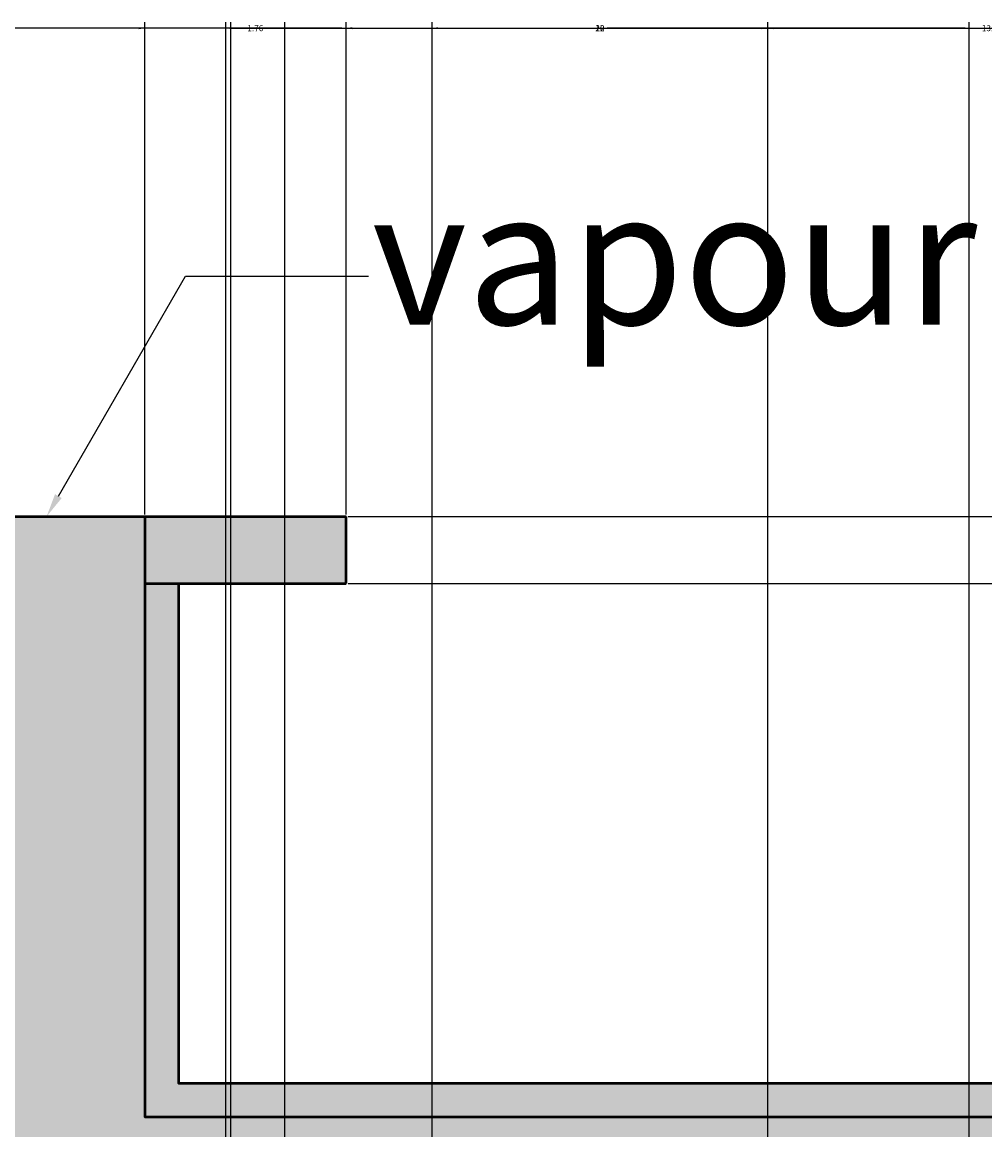
# Model space of a CAD drawing. Units: inches. Extents: x -12 to 334, y -10 to 186.
# Tile 67 of 77: x 210 to 239, y 137 to 170. Entities that reach past the tile are written whole.
import ezdxf
from ezdxf import colors
from ezdxf.entities.mleader import LeaderData, LeaderLine
from ezdxf.math import Vec2, Vec3

# ---------------------------------------------------------------- set-up
doc = ezdxf.new("R2010")
doc.units = ezdxf.units.IN
doc.header["$MEASUREMENT"] = 0
for name, color, linetype, lineweight in [('M-ANNO-TEXT', 3, 'Continuous', 25), ('M-DIMS', 2, 'Continuous', 18), ('M-EQPM', 7, 'Continuous', 50), ('M-EQPM-PATT', 8, 'Continuous', 18)]:
    doc.layers.add(name, color=color, linetype=linetype, lineweight=lineweight)
doc.styles.get("Standard").update_dxf_attribs({"font": 'arial.ttf'})
doc.dimstyles.get("Standard").update_dxf_attribs({"dimtxt": 0.18, "dimasz": 0.18, "dimexe": 0.18, "dimexo": 0.0625, "dimgap": 0.09, "dimtad": 0, "dimtih": 1, "dimtoh": 1, "dimdec": 4, "dimzin": 0, "dimdsep": 46, "dimtxsty": 'Standard', "dimcen": 0.09, "dimadec": 0, "dimazin": 0, "dimtfac": 1, "dimtdec": 4, "dimtofl": 0, "dimtmove": 0, "dimatfit": 3, "dimfxl": 1, "dimtolj": 1, "dimtzin": 0, "dimarcsym": 0})

# ---------------------------------------------------------------- blocks, each defined once
blk = doc.blocks.new('*D19')
at = {"layer": 'Defpoints', "color": 0, "transparency": 16777216}
for p in [(220.017, 169.385), (190.342, 154.835), (220.017, 154.835)]:
    blk.add_point(p, dxfattribs=at)
at = {"layer": 'M-DIMS', "color": 0, "lineweight": -2, "transparency": 16777216}
for p, q in [((190.342, 154.897), (190.342, 169.565)), ((190.522, 169.385), (204.714, 169.385)), ((219.837, 169.385), (205.645, 169.385)), ((220.017, 154.897), (220.017, 169.565))]:
    blk.add_line(p, q, dxfattribs=at)
at = {"layer": 'M-DIMS', "color": 0, "transparency": 16777216}
for points in [[(190.522, 169.415), (190.522, 169.355), (190.342, 169.385)], [(219.837, 169.415), (219.837, 169.355), (220.017, 169.385)]]:
    blk.add_solid(points, dxfattribs=at)
at = {"layer": 'M-DIMS', "color": 0, "transparency": 16777216, "insert": (205.179, 169.385), "char_height": 0.18, "attachment_point": 5}
blk.add_mtext('\\A1;29.675', dxfattribs=at)
blk = doc.blocks.new('*D20')
at = {"layer": 'Defpoints', "color": 0, "transparency": 16777216}
for p in [(214.017, 169.385), (196.342, 154.835), (214.017, 154.835)]:
    blk.add_point(p, dxfattribs=at)
at = {"layer": 'M-DIMS', "color": 0, "lineweight": -2, "transparency": 16777216}
for p, q in [((196.342, 154.897), (196.342, 169.565)), ((196.522, 169.385), (204.724, 169.385)), ((213.837, 169.385), (205.635, 169.385)), ((214.017, 154.897), (214.017, 169.565))]:
    blk.add_line(p, q, dxfattribs=at)
at = {"layer": 'M-DIMS', "color": 0, "transparency": 16777216}
for points in [[(196.522, 169.415), (196.522, 169.355), (196.342, 169.385)], [(213.837, 169.415), (213.837, 169.355), (214.017, 169.385)]]:
    blk.add_solid(points, dxfattribs=at)
at = {"layer": 'M-DIMS', "color": 0, "transparency": 16777216, "insert": (205.179, 169.385), "char_height": 0.18, "attachment_point": 5}
blk.add_mtext('\\A1;17.675', dxfattribs=at)
blk = doc.blocks.new('*D21')
at = {"layer": 'Defpoints', "color": 0, "transparency": 16777216}
for p in [(269.381, 169.385), (220.017, 154.835), (269.381, 137.943)]:
    blk.add_point(p, dxfattribs=at)
at = {"layer": 'M-DIMS', "color": 0, "lineweight": -2, "transparency": 16777216}
for p, q in [((220.017, 154.897), (220.017, 169.565)), ((220.197, 169.385), (244.301, 169.385)), ((269.201, 169.385), (245.096, 169.385)), ((269.381, 138.006), (269.381, 169.565))]:
    blk.add_line(p, q, dxfattribs=at)
at = {"layer": 'M-DIMS', "color": 0, "transparency": 16777216}
for points in [[(220.197, 169.415), (220.197, 169.355), (220.017, 169.385)], [(269.201, 169.415), (269.201, 169.355), (269.381, 169.385)]]:
    blk.add_solid(points, dxfattribs=at)
at = {"layer": 'M-DIMS', "color": 0, "transparency": 16777216, "insert": (244.699, 169.385), "char_height": 0.18, "attachment_point": 5}
blk.add_mtext('\\A1;49.36', dxfattribs=at)
blk = doc.blocks.new('*D23')
at = {"layer": 'Defpoints', "color": 0, "transparency": 16777216}
for p in [(220.017, 154.835), (220.017, 152.835), (295.976, 152.835)]:
    blk.add_point(p, dxfattribs=at)
at = {"layer": 'M-DIMS', "color": 0, "lineweight": -2, "transparency": 16777216}
for p, q in [((220.079, 154.835), (296.156, 154.835)), ((295.976, 154.655), (295.976, 154.015)), ((295.976, 153.015), (295.976, 153.654)), ((220.079, 152.835), (296.156, 152.835))]:
    blk.add_line(p, q, dxfattribs=at)
at = {"layer": 'M-DIMS', "color": 0, "transparency": 16777216}
for points in [[(295.946, 154.655), (296.006, 154.655), (295.976, 154.835)], [(295.946, 153.015), (296.006, 153.015), (295.976, 152.835)]]:
    blk.add_solid(points, dxfattribs=at)
at = {"layer": 'M-DIMS', "color": 0, "transparency": 16777216, "insert": (295.976, 153.835), "char_height": 0.18, "attachment_point": 5}
blk.add_mtext('\\A1;2', dxfattribs=at)
blk = doc.blocks.new('*D27')
at = {"layer": 'Defpoints', "color": 0, "transparency": 16777216}
for p in [(238.576, 169.385), (216.576, 32.854), (238.576, 32.854)]:
    blk.add_point(p, dxfattribs=at)
at = {"layer": 'M-DIMS', "color": 0, "lineweight": -2, "transparency": 16777216}
for p, q in [((216.576, 32.917), (216.576, 169.565)), ((216.756, 169.385), (227.357, 169.385)), ((238.396, 169.385), (227.796, 169.385)), ((238.576, 32.917), (238.576, 169.565))]:
    blk.add_line(p, q, dxfattribs=at)
at = {"layer": 'M-DIMS', "color": 0, "transparency": 16777216}
for points in [[(216.756, 169.415), (216.756, 169.355), (216.576, 169.385)], [(238.396, 169.415), (238.396, 169.355), (238.576, 169.385)]]:
    blk.add_solid(points, dxfattribs=at)
at = {"layer": 'M-DIMS', "color": 0, "transparency": 16777216, "insert": (227.576, 169.385), "char_height": 0.18, "attachment_point": 5}
blk.add_mtext('\\A1;22', dxfattribs=at)
blk = doc.blocks.new('*D28')
at = {"layer": 'Defpoints', "color": 0, "transparency": 16777216}
for p in [(232.576, 169.385), (222.576, 30.854), (232.576, 30.854)]:
    blk.add_point(p, dxfattribs=at)
at = {"layer": 'M-DIMS', "color": 0, "lineweight": -2, "transparency": 16777216}
for p, q in [((222.576, 30.917), (222.576, 169.565)), ((222.756, 169.385), (227.366, 169.385)), ((232.396, 169.385), (227.786, 169.385)), ((232.576, 30.917), (232.576, 169.565))]:
    blk.add_line(p, q, dxfattribs=at)
at = {"layer": 'M-DIMS', "color": 0, "transparency": 16777216}
for points in [[(222.756, 169.415), (222.756, 169.355), (222.576, 169.385)], [(232.396, 169.415), (232.396, 169.355), (232.576, 169.385)]]:
    blk.add_solid(points, dxfattribs=at)
at = {"layer": 'M-DIMS', "color": 0, "transparency": 16777216, "insert": (227.576, 169.385), "char_height": 0.18, "attachment_point": 5}
blk.add_mtext('\\A1;10', dxfattribs=at)
blk = doc.blocks.new('*D34')
at = {"layer": 'Defpoints', "color": 0, "transparency": 16777216}
for p in [(218.192, 169.385), (216.428, 98.108), (218.192, 98.108)]:
    blk.add_point(p, dxfattribs=at)
at = {"layer": 'M-DIMS', "color": 0, "lineweight": -2, "transparency": 16777216}
for p, q in [((216.428, 98.171), (216.428, 169.565)), ((216.608, 169.385), (216.995, 169.385)), ((218.012, 169.385), (217.625, 169.385)), ((218.192, 98.171), (218.192, 169.565))]:
    blk.add_line(p, q, dxfattribs=at)
at = {"layer": 'M-DIMS', "color": 0, "transparency": 16777216}
for points in [[(216.608, 169.415), (216.608, 169.355), (216.428, 169.385)], [(218.012, 169.415), (218.012, 169.355), (218.192, 169.385)]]:
    blk.add_solid(points, dxfattribs=at)
at = {"layer": 'M-DIMS', "color": 0, "transparency": 16777216, "insert": (217.31, 169.385), "char_height": 0.18, "attachment_point": 5}
blk.add_mtext('\\A1;1.76', dxfattribs=at)
blk = doc.blocks.new('*D37')
at = {"layer": 'Defpoints', "color": 0, "transparency": 16777216}
for p in [(245.935, 169.385), (232.576, 46.854), (245.935, 46.854)]:
    blk.add_point(p, dxfattribs=at)
at = {"layer": 'M-DIMS', "color": 0, "lineweight": -2, "transparency": 16777216}
for p, q in [((232.576, 46.917), (232.576, 169.565)), ((232.756, 169.385), (238.871, 169.385)), ((245.755, 169.385), (239.641, 169.385)), ((245.935, 46.917), (245.935, 169.565))]:
    blk.add_line(p, q, dxfattribs=at)
at = {"layer": 'M-DIMS', "color": 0, "transparency": 16777216}
for points in [[(232.756, 169.415), (232.756, 169.355), (232.576, 169.385)], [(245.755, 169.415), (245.755, 169.355), (245.935, 169.385)]]:
    blk.add_solid(points, dxfattribs=at)
at = {"layer": 'M-DIMS', "color": 0, "transparency": 16777216, "insert": (239.256, 169.385), "char_height": 0.18, "attachment_point": 5}
blk.add_mtext('\\A1;13.36', dxfattribs=at)

msp = doc.modelspace()

# ---------------------------------------------------------------- hatches: boundary and pattern name
at = {"layer": 'M-EQPM-PATT', "transparency": 33554556}
h = msp.add_hatch(color=256, dxfattribs=at)
h.set_gradient(color1=(248, 206, 179), color2=(248, 206, 179), tint=1)
h.paths.add_polyline_path([(179.7818, 136.8871), (126.9567, 136.8871), (106.1771, 100.8958), (171.5458, 100.8958)])
h.paths.add_polyline_path([(268.3808, 136.9435), (214.0166, 136.9435), (214.0166, 154.8345), (196.3421, 154.8345), (196.3421, 136.8871), (179.7818, 136.8871), (171.5458, 100.8958), (231.7758, 100.8958, -0.4142136), (251.9801, 80.6915), (279.7263, 80.6915, 0.1631825)])
at = {"layer": 'M-EQPM-PATT'}
h = msp.add_hatch(color=256, dxfattribs=at)
h.set_gradient(color1=(99, 100, 102), color2=(99, 100, 102), tint=1)
h.paths.add_polyline_path([(190.3421, 154.8345), (190.3421, 152.8345), (196.3421, 152.8345), (196.3421, 154.8345)])
h.paths.add_polyline_path([(220.0166, 152.8345), (220.0166, 154.8345), (214.0166, 154.8345), (214.0166, 152.8345)])
h = msp.add_hatch(color=256, dxfattribs=at)
h.set_gradient(color1=(99, 100, 102), color2=(99, 100, 102), tint=1)
h.paths.add_polyline_path([(126.9567, 136.8871), (179.7818, 136.8871), (180.0106, 137.8871), (126.3793, 137.8871), (106.1771, 102.8958), (86.8879, 102.8958), (86.8879, 109.0583), (84.7229, 109.0583), (84.7229, 100.8958), (106.1771, 100.8958)])
h.paths.add_polyline_path([(196.3421, 152.8345), (195.3421, 152.8345), (195.3421, 137.8871), (180.0106, 137.8871), (179.7818, 136.8871), (196.3421, 136.8871)])
h.paths.add_polyline_path([(215.0166, 152.8345), (214.0166, 152.8345), (214.0166, 136.9435), (268.3808, 136.9435, -0.2673785), (268.3808, 46.8541), (249.3759, 46.8541), (249.8485, 45.8541), (269.3808, 45.8541, 0.2615891), (269.3808, 137.9435), (215.0166, 137.9435)])

# ---------------------------------------------------------------- linework, layer by layer
at = {"layer": 'M-EQPM'}
for p, q in [((190.3421, 154.8345), (220.0166, 154.8345)), ((220.0166, 152.8345), (220.0166, 154.8345)), ((214.0166, 152.8345), (220.0166, 152.8345))]:
    msp.add_line(p, q, dxfattribs=at)
for points in [[(214.0166, 154.8345), (214.0166, 136.9435), (268.3808, 136.9435)], [(215.0166, 152.8345), (215.0166, 137.9435), (269.3808, 137.9435)]]:
    msp.add_lwpolyline(points, dxfattribs=at)

# ---------------------------------------------------------------- dimensions: what is measured, and where the dimension line sits
at = {"layer": 'M-DIMS'}
for base, p1, p2, override, picture, middle in [((220.01662, 169.38453), (190.34209, 154.83453), (220.01662, 154.83453), {"dimdec": 3, "dimlfac": 1, "dimrnd": 0, "dimzin": 0, "dimdsep": 46, "dimlunit": 2}, '*D19', (205.17936, 169.38453)), ((214.01662, 169.38453), (196.34209, 154.83453), (214.01662, 154.83453), {"dimdec": 3, "dimlfac": 1, "dimrnd": 0, "dimzin": 0, "dimdsep": 46, "dimlunit": 2}, '*D20', (205.17936, 169.38453)), ((218.1922, 169.3845), (216.4278, 98.1081), (218.1922, 98.1081), {"dimdec": 2, "dimlfac": 1, "dimrnd": 0, "dimzin": 0, "dimdsep": 46, "dimlunit": 2}, '*D34', (217.31, 169.3845)), ((238.5761, 169.3845), (216.5761, 32.8541), (238.5761, 32.8541), {"dimdec": 0, "dimlfac": 1, "dimrnd": 0, "dimzin": 0, "dimdsep": 46, "dimlunit": 2}, '*D27', (227.5761, 169.3845)), ((269.3808, 169.3845), (220.0166, 154.8345), (269.3808, 137.9435), {"dimdec": 2, "dimlfac": 1, "dimrnd": 0, "dimzin": 0, "dimdsep": 46, "dimlunit": 2}, '*D21', (244.6987, 169.3845)), ((232.5761, 169.3845), (222.5761, 30.8541), (232.5761, 30.8541), {"dimdec": 0, "dimlfac": 1, "dimrnd": 0, "dimzin": 0, "dimdsep": 46, "dimlunit": 2}, '*D28', (227.5761, 169.3845)), ((245.9354, 169.3845), (232.5761, 46.8541), (245.9354, 46.8541), {"dimdec": 2, "dimlfac": 1, "dimrnd": 0, "dimzin": 0, "dimdsep": 46, "dimlunit": 2}, '*D37', (239.2558, 169.3845))]:
    dim = msp.add_linear_dim(base=base, p1=p1, p2=p2, dimstyle='Standard', override=override, dxfattribs=at)
    dim.commit()
    dim.dimension.update_dxf_attribs({"geometry": picture, "text_midpoint": middle})
dim = msp.add_linear_dim(base=(295.9756, 152.8345), p1=(220.0166, 154.8345), p2=(220.0166, 152.8345), angle=90, dimstyle='Standard', override={"dimdec": 0, "dimlfac": 1, "dimrnd": 0, "dimzin": 0, "dimdsep": 46, "dimlunit": 2}, dxfattribs=at)
dim.commit()
dim.dimension.update_dxf_attribs({"geometry": '*D23', "text_midpoint": (295.9756, 153.8345)})

# ---------------------------------------------------------------- leaders
at = {"layer": 'M-ANNO-TEXT'}
ml = msp.add_multileader_mtext('Standard', dxfattribs=at)
ml.set_content('vapour outlet to column', color=256)
ml.set_leader_properties()
ml.build(insert=Vec2(0, 0))
ml.multileader.update_dxf_attribs({"dogleg_length": 0.36, "arrow_head_size": 0.7})
ctx = ml.context
ctx.base_point, ctx.arrow_head_size, ctx.landing_gap_size, ctx.plane_origin = Vec3(220.6842, 161.9963), 0.7, 0.09, Vec3(211.0929, 154.8345)
notes = []
notes.append((ctx, [(0, (1, 1, 0), (215.2277, 161.9963), (1, 0), 5.4565, [(0, [(211.0929, 154.8345)], 0, [])])]))
ctx.mtext.insert, ctx.mtext.flow_direction = Vec3(220.7742, 164.5515), 5
for ctx, leaders in notes:
    for number, flags, end, landing, length, lines in leaders:
        leader = LeaderData()
        leader.index, (leader.has_last_leader_line, leader.has_dogleg_vector, leader.attachment_direction) = number, flags
        leader.last_leader_point, leader.dogleg_vector, leader.dogleg_length = Vec3(end), Vec3(landing), length
        for number, points, colour, breaks in lines:
            line = LeaderLine()
            line.index, line.vertices, line.color, line.breaks = number, Vec3.list(points), colors.encode_raw_color(colour), breaks
            leader.lines.append(line)
        ctx.leaders.append(leader)

doc.saveas('drawing.dxf')
